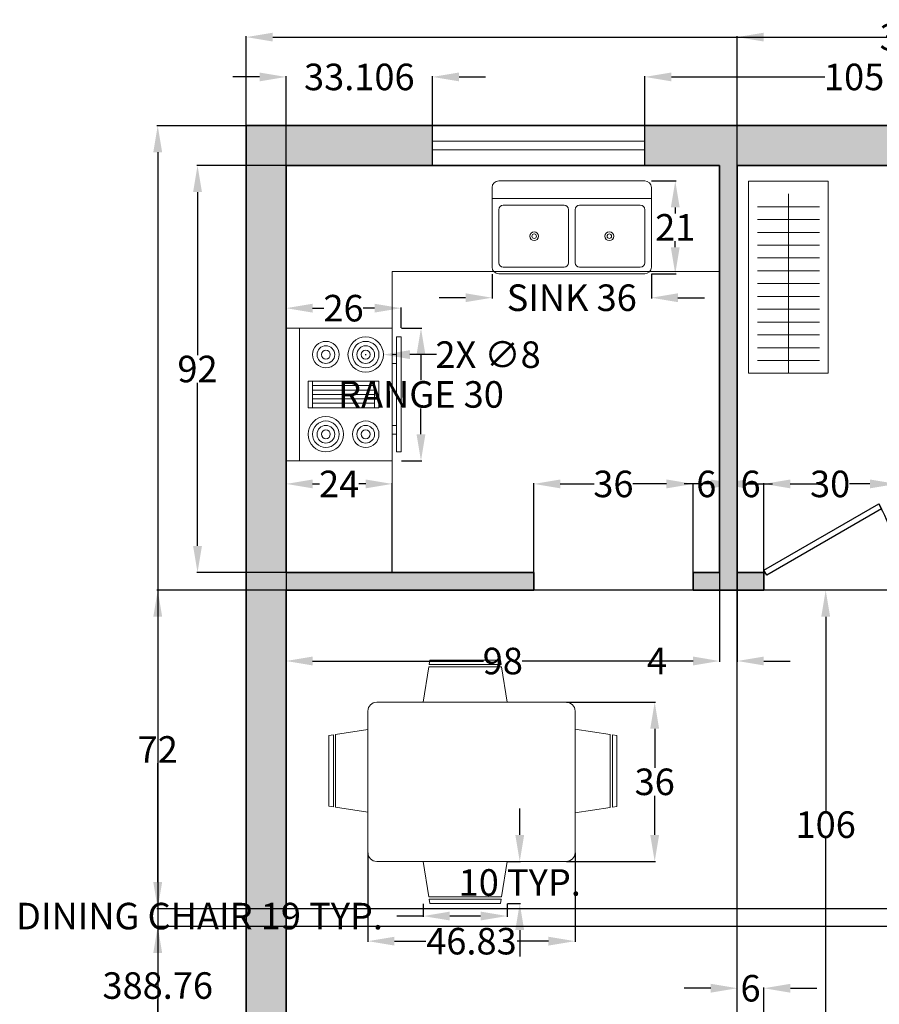
# Model space of a CAD drawing. Units: inches. Extents: x -26 to 363, y -399 to 37.
# Tile 3 of 4: x -26 to 168, y -185 to 37. Entities that reach past the tile are written whole.
import ezdxf

# ---------------------------------------------------------------- set-up
doc = ezdxf.new("R2010")
doc.units = ezdxf.units.IN
doc.header["$MEASUREMENT"] = 0
for name, color, linetype, lineweight in [('A-ANNO-DIMS', 2, 'Continuous', 18), ('A-DOOR', 3, 'Continuous', 25), ('A-EQPM', 9, 'Continuous', 18), ('A-FLOR-CASE', 8, 'Continuous', 18), ('A-FLOR-FIXT', 9, 'Continuous', 18), ('A-FURN', 8, 'Continuous', 18), ('A-GLAZ', 4, 'Continuous', 18), ('A-WALL', 7, 'Continuous', 35), ('A-WALL-PATT', 251, 'Continuous', 13)]:
    doc.layers.add(name, color=color, linetype=linetype, lineweight=lineweight)
doc.styles.get("Standard").update_dxf_attribs({"font": 'arial.ttf'})
doc.dimstyles.get("Standard").update_dxf_attribs({"dimtxt": 6, "dimasz": 6, "dimexe": 0.18, "dimexo": 0.0625, "dimgap": 0.09, "dimtad": 0, "dimtih": 1, "dimtoh": 1, "dimdec": 0, "dimzin": 0, "dimdsep": 46, "dimlunit": 4, "dimtxsty": 'Standard', "dimcen": 0.09, "dimadec": 0, "dimazin": 0, "dimtfac": 1, "dimtdec": 0, "dimtofl": 0, "dimtmove": 0, "dimatfit": 3, "dimfxl": 1, "dimtolj": 1, "dimtzin": 0, "dimarcsym": 0})

# ---------------------------------------------------------------- blocks, each defined once
blk = doc.blocks.new('*U2')
for p, q in [((0, 0), (0, -6)), ((40, 0), (40, -6))]:
    blk.add_line(p, q)
blk.add_lwpolyline([(0, 0), (34.64, 20), (35.52, 18.48), (0.87, -1.52)], close=True)
blk.add_arc((0, 0), 40, 0, 30)
blk = doc.blocks.new('Range-Oven - 30 in top')
for p, q in [((0, -3), (30, -3)), ((12, -6), (18, -6)), ((13, -20), (13, -6)), ((14, -6), (14, -20)), ((15, -20), (15, -6)), ((16, -6), (16, -20)), ((17, -20), (17, -6)), ((18, -20), (12, -20)), ((6, -24), (6, -25)), ((8, -25), (8, -24)), ((22, -25), (22, -24)), ((24, -24), (24, -25))]:
    blk.add_line(p, q)
for points in [[(0, -24), (0, 0), (30, 0), (30, -24)], [(12, -21), (12, -5), (18, -5), (18, -21)], [(2, -26), (2, -25), (28, -25), (28, -26)]]:
    blk.add_lwpolyline(points, close=True)
for centre, radius in [((6, -9), 4), ((6, -9), 3), ((24, -9), 3), ((6, -9), 2), ((6, -9), 1), ((24, -9), 2), ((24, -9), 1), ((6, -18), 3), ((24, -18), 4), ((24, -18), 3), ((6, -18), 2), ((6, -18), 1), ((24, -18), 2), ((24, -18), 1)]:
    blk.add_circle(centre, radius)
blk = doc.blocks.new('Sink-double - 36 in top')
for p, q in [((-18, -4), (18, -4)), ((-0.75, -18.5), (-0.75, -6.5)), ((0.75, -6.5), (0.75, -18.5))]:
    blk.add_line(p, q)
for points in [[(-16.5, 0), (16.5, 0)], [(-18, -19.5), (-18, -1.5)], [(18, -1.5), (18, -19.5)], [(-16.5, -18.5), (-16.5, -6.5)], [(-15.5, -5.5), (-1.75, -5.5)], [(1.75, -5.5), (15.5, -5.5)], [(16.5, -6.5), (16.5, -18.5)], [(-1.75, -19.5), (-15.5, -19.5)], [(15.5, -19.5), (1.75, -19.5)], [(16.5, -21), (-16.5, -21)]]:
    blk.add_lwpolyline(points)
for centre, radius in [((-8.5, -12.5), 1), ((-8.5, -12.5), 0.5), ((8.5, -12.5), 1), ((8.5, -12.5), 0.5)]:
    blk.add_circle(centre, radius)
for centre, radius, start, end in [((-16.5, -1.5), 1.5, 90, 180), ((16.5, -1.5), 1.5, 0, 90), ((-15.5, -6.5), 1, 90, 180), ((-1.75, -6.5), 1, 0, 90), ((1.75, -6.5), 1, 90, 180), ((15.5, -6.5), 1, 0, 90), ((-16.5, -19.5), 1.5, 180, 270), ((-15.5, -18.5), 1, 180, 270), ((-1.75, -18.5), 1, 270, 0), ((1.75, -18.5), 1, 180, 270), ((15.5, -18.5), 1, 270, 0), ((16.5, -19.5), 1.5, 270, 0)]:
    blk.add_arc(centre, radius, start, end)
blk = doc.blocks.new('WIN-48IN')
for p, q in [((0, 0), (0, 9)), ((48, 9), (48, 0)), ((48, 5.5), (0, 5.5)), ((48, 3.5), (0, 3.5))]:
    blk.add_line(p, q)
blk = doc.blocks.new('CHAIR-DINING')
for p, q in [((1.48, 9.5), (1.33, 8.5)), ((1.48, 9.5), (17.48, 9.5)), ((17.64, 8.5), (17.48, 9.5)), ((1.25, 8), (0, 0)), ((1.25, 8), (17.72, 8)), ((17.64, 8.5), (1.33, 8.5)), ((18.97, 0), (17.72, 8))]:
    blk.add_line(p, q)
blk = doc.blocks.new('*D25')
at = {"layer": 'A-ANNO-DIMS', "color": 0, "lineweight": -2, "transparency": 16777216}
for p, q in [((65.33, -162.44), (65.33, -165.41)), ((84.3, -162.44), (84.3, -165.4)), ((65.33, -165.23), (59.33, -165.23)), ((78.3, -165.22), (71.33, -165.22))]:
    blk.add_line(p, q, dxfattribs=at)
at = {"layer": 'A-ANNO-DIMS', "color": 0, "transparency": 16777216}
for points in [[(71.33, -164.22), (71.33, -166.22), (65.33, -165.23)], [(78.3, -164.22), (78.3, -166.22), (84.3, -165.22)]]:
    blk.add_solid(points, dxfattribs=at)
at = {"layer": 'Defpoints', "color": 0, "transparency": 16777216}
for p in [(65.33, -162.38), (84.3, -162.38), (65.33, -165.23)]:
    blk.add_point(p, dxfattribs=at)
at = {"layer": 'A-ANNO-DIMS', "color": 0, "transparency": 16777216, "insert": (14.75, -165.23), "char_height": 6, "attachment_point": 5}
blk.add_mtext('\\A1;DINING CHAIR 19 TYP.', dxfattribs=at)
blk = doc.blocks.new('*D26')
at = {"layer": 'A-ANNO-DIMS', "color": 0, "lineweight": -2, "transparency": 16777216}
for p, q in [((87.15, -146.88), (87.15, -140.88)), ((84.36, -152.88), (87.33, -152.88)), ((84.36, -162.38), (87.33, -162.38)), ((87.15, -168.38), (87.15, -174.38))]:
    blk.add_line(p, q, dxfattribs=at)
at = {"layer": 'A-ANNO-DIMS', "color": 0, "transparency": 16777216}
for points in [[(88.15, -146.88), (86.15, -146.88), (87.15, -152.88)], [(88.15, -168.38), (86.15, -168.38), (87.15, -162.38)]]:
    blk.add_solid(points, dxfattribs=at)
at = {"layer": 'Defpoints', "color": 0, "transparency": 16777216}
for p in [(84.3, -152.88), (84.3, -162.38), (87.15, -162.38)]:
    blk.add_point(p, dxfattribs=at)
at = {"layer": 'A-ANNO-DIMS', "color": 0, "transparency": 16777216, "insert": (87.15, -157.63), "char_height": 6, "attachment_point": 5}
blk.add_mtext('\\A1;10 TYP.', dxfattribs=at)
blk = doc.blocks.new('*D33')
at = {"layer": 'A-ANNO-DIMS', "color": 0, "lineweight": -2, "transparency": 16777216}
for p, q in [((60.39, -32.31), (65, -32.31)), ((64.82, -38.31), (64.82, -44.12)), ((64.82, -56.31), (64.82, -50.51)), ((60.39, -62.31), (65, -62.31))]:
    blk.add_line(p, q, dxfattribs=at)
at = {"layer": 'A-ANNO-DIMS', "color": 0, "transparency": 16777216}
for points in [[(63.82, -38.31), (65.82, -38.31), (64.82, -32.31)], [(63.82, -56.31), (65.82, -56.31), (64.82, -62.31)]]:
    blk.add_solid(points, dxfattribs=at)
at = {"layer": 'Defpoints', "color": 0, "transparency": 16777216}
for p in [(60.32, -32.31), (64.82, -32.31), (60.32, -62.31)]:
    blk.add_point(p, dxfattribs=at)
at = {"layer": 'A-ANNO-DIMS', "color": 0, "transparency": 16777216, "insert": (64.82, -47.31), "char_height": 6, "attachment_point": 5}
blk.add_mtext('\\A1;RANGE 30', dxfattribs=at)
blk = doc.blocks.new('*D34')
at = {"layer": 'A-ANNO-DIMS', "color": 0, "lineweight": -2, "transparency": 16777216}
for p, q in [((34.32, -32.25), (34.32, -27.63)), ((40.32, -27.81), (42.89, -27.81)), ((54.32, -27.81), (51.76, -27.81)), ((60.32, -32.25), (60.32, -27.63))]:
    blk.add_line(p, q, dxfattribs=at)
at = {"layer": 'A-ANNO-DIMS', "color": 0, "transparency": 16777216}
for points in [[(40.32, -26.81), (40.32, -28.81), (34.32, -27.81)], [(54.32, -26.81), (54.32, -28.81), (60.32, -27.81)]]:
    blk.add_solid(points, dxfattribs=at)
at = {"layer": 'Defpoints', "color": 0, "transparency": 16777216}
for p in [(34.32, -27.81), (34.32, -32.31), (60.32, -32.31)]:
    blk.add_point(p, dxfattribs=at)
at = {"layer": 'A-ANNO-DIMS', "color": 0, "transparency": 16777216, "insert": (47.32, -27.81), "char_height": 6, "attachment_point": 5}
blk.add_mtext('\\A1;26', dxfattribs=at)
blk = doc.blocks.new('*D35')
at = {"layer": 'A-ANNO-DIMS', "color": 0, "lineweight": -2, "transparency": 16777216}
for p, q in [((80.91, -20.11), (80.91, -25.63)), ((116.91, -20.11), (116.91, -25.63)), ((74.91, -25.45), (68.91, -25.45)), ((122.91, -25.45), (128.91, -25.45))]:
    blk.add_line(p, q, dxfattribs=at)
at = {"layer": 'A-ANNO-DIMS', "color": 0, "transparency": 16777216}
for points in [[(74.91, -24.45), (74.91, -26.45), (80.91, -25.45)], [(122.91, -24.45), (122.91, -26.45), (116.91, -25.45)]]:
    blk.add_solid(points, dxfattribs=at)
at = {"layer": 'Defpoints', "color": 0, "transparency": 16777216}
for p in [(80.91, -20.05), (116.91, -20.05), (116.91, -25.45)]:
    blk.add_point(p, dxfattribs=at)
at = {"layer": 'A-ANNO-DIMS', "color": 0, "transparency": 16777216, "insert": (98.91, -25.45), "char_height": 6, "attachment_point": 5}
blk.add_mtext('\\A1;SINK 36', dxfattribs=at)
blk = doc.blocks.new('*D36')
at = {"layer": 'A-ANNO-DIMS', "color": 0, "lineweight": -2, "transparency": 16777216}
for p, q in [((116.97, 0.95), (122.49, 0.95)), ((122.31, -5.05), (122.31, -6.44)), ((122.31, -14.05), (122.31, -12.65)), ((116.97, -20.05), (122.49, -20.05))]:
    blk.add_line(p, q, dxfattribs=at)
at = {"layer": 'A-ANNO-DIMS', "color": 0, "transparency": 16777216}
for points in [[(121.31, -5.05), (123.31, -5.05), (122.31, 0.95)], [(121.31, -14.05), (123.31, -14.05), (122.31, -20.05)]]:
    blk.add_solid(points, dxfattribs=at)
at = {"layer": 'Defpoints', "color": 0, "transparency": 16777216}
for p in [(116.91, 0.95), (122.31, 0.95), (116.91, -20.05)]:
    blk.add_point(p, dxfattribs=at)
at = {"layer": 'A-ANNO-DIMS', "color": 0, "transparency": 16777216, "insert": (122.31, -9.55), "char_height": 6, "attachment_point": 5}
blk.add_mtext('\\A1;21', dxfattribs=at)
blk = doc.blocks.new('*D39')
at = {"layer": 'A-ANNO-DIMS', "color": 0, "lineweight": -2, "transparency": 16777216}
for p, q in [((25.32, 13.51), (25.32, 33.64)), ((31.32, 33.46), (168.62, 33.46)), ((319.32, 33.46), (182.03, 33.46)), ((325.32, 13.51), (325.32, 33.64))]:
    blk.add_line(p, q, dxfattribs=at)
at = {"layer": 'A-ANNO-DIMS', "color": 0, "transparency": 16777216}
for points in [[(31.32, 34.46), (31.32, 32.46), (25.32, 33.46)], [(319.32, 34.46), (319.32, 32.46), (325.32, 33.46)]]:
    blk.add_solid(points, dxfattribs=at)
at = {"layer": 'Defpoints', "color": 0, "transparency": 16777216}
for p in [(325.32, 33.46), (25.32, 13.44), (325.32, 13.44)]:
    blk.add_point(p, dxfattribs=at)
at = {"layer": 'A-ANNO-DIMS', "color": 0, "transparency": 16777216, "insert": (175.32, 33.46), "char_height": 6, "attachment_point": 5}
blk.add_mtext('\\A1;300', dxfattribs=at)
blk = doc.blocks.new('*D40')
at = {"layer": 'A-ANNO-DIMS', "color": 0, "lineweight": -2, "transparency": 16777216}
for p, q in [((25.26, 13.44), (5.13, 13.44)), ((5.31, 7.44), (5.31, -177.78)), ((5.31, -369.31), (5.31, -184.09)), ((76.26, -375.31), (5.13, -375.31))]:
    blk.add_line(p, q, dxfattribs=at)
at = {"layer": 'A-ANNO-DIMS', "color": 0, "transparency": 16777216}
for points in [[(4.31, 7.44), (6.31, 7.44), (5.31, 13.44)], [(4.31, -369.31), (6.31, -369.31), (5.31, -375.31)]]:
    blk.add_solid(points, dxfattribs=at)
at = {"layer": 'Defpoints', "color": 0, "transparency": 16777216}
for p in [(25.32, 13.44), (5.31, -375.31), (76.32, -375.31)]:
    blk.add_point(p, dxfattribs=at)
at = {"layer": 'A-ANNO-DIMS', "color": 0, "transparency": 16777216, "insert": (5.31, -180.93), "char_height": 6, "attachment_point": 5}
blk.add_mtext('\\A1;388.76', dxfattribs=at)
blk = doc.blocks.new('*D45')
at = {"layer": 'A-ANNO-DIMS', "color": 0, "lineweight": -2, "transparency": 16777216}
for p, q in [((34.32, -87.62), (34.32, -107.75)), ((132.32, -87.62), (132.32, -107.75)), ((40.32, -107.57), (78.93, -107.57)), ((126.32, -107.57), (87.72, -107.57))]:
    blk.add_line(p, q, dxfattribs=at)
at = {"layer": 'A-ANNO-DIMS', "color": 0, "transparency": 16777216}
for points in [[(40.32, -106.57), (40.32, -108.57), (34.32, -107.57)], [(126.32, -106.57), (126.32, -108.57), (132.32, -107.57)]]:
    blk.add_solid(points, dxfattribs=at)
at = {"layer": 'Defpoints', "color": 0, "transparency": 16777216}
for p in [(34.32, -87.56), (132.32, -87.56), (34.32, -107.57)]:
    blk.add_point(p, dxfattribs=at)
at = {"layer": 'A-ANNO-DIMS', "color": 0, "transparency": 16777216, "insert": (83.32, -107.57), "char_height": 6, "attachment_point": 5}
blk.add_mtext('\\A1;98', dxfattribs=at)
blk = doc.blocks.new('*D46')
at = {"layer": 'A-ANNO-DIMS', "color": 0, "lineweight": -2, "transparency": 16777216}
for p, q in [((34.26, 4.44), (14.13, 4.44)), ((14.31, -1.56), (14.31, -38.4)), ((14.31, -81.56), (14.31, -44.71)), ((34.26, -87.56), (14.13, -87.56))]:
    blk.add_line(p, q, dxfattribs=at)
at = {"layer": 'A-ANNO-DIMS', "color": 0, "transparency": 16777216}
for points in [[(13.31, -1.56), (15.31, -1.56), (14.31, 4.44)], [(13.31, -81.56), (15.31, -81.56), (14.31, -87.56)]]:
    blk.add_solid(points, dxfattribs=at)
at = {"layer": 'Defpoints', "color": 0, "transparency": 16777216}
for p in [(14.31, 4.44), (34.32, 4.44), (34.32, -87.56)]:
    blk.add_point(p, dxfattribs=at)
at = {"layer": 'A-ANNO-DIMS', "color": 0, "transparency": 16777216, "insert": (14.31, -41.56), "char_height": 6, "attachment_point": 5}
blk.add_mtext('\\A1;92', dxfattribs=at)
blk = doc.blocks.new('*D48')
at = {"layer": 'A-ANNO-DIMS', "color": 0, "lineweight": -2, "transparency": 16777216}
for p, q in [((176.26, -91.56), (156.13, -91.56)), ((156.31, -97.56), (156.31, -141.4)), ((156.31, -191.56), (156.31, -147.71)), ((176.26, -197.56), (156.13, -197.56))]:
    blk.add_line(p, q, dxfattribs=at)
at = {"layer": 'A-ANNO-DIMS', "color": 0, "transparency": 16777216}
for points in [[(155.31, -97.56), (157.31, -97.56), (156.31, -91.56)], [(155.31, -191.56), (157.31, -191.56), (156.31, -197.56)]]:
    blk.add_solid(points, dxfattribs=at)
at = {"layer": 'Defpoints', "color": 0, "transparency": 16777216}
for p in [(156.31, -91.56), (176.32, -91.56), (176.32, -197.56)]:
    blk.add_point(p, dxfattribs=at)
at = {"layer": 'A-ANNO-DIMS', "color": 0, "transparency": 16777216, "insert": (156.31, -144.56), "char_height": 6, "attachment_point": 5}
blk.add_mtext('\\A1;106', dxfattribs=at)
blk = doc.blocks.new('*D50')
at = {"layer": 'A-ANNO-DIMS', "color": 0, "lineweight": -2, "transparency": 16777216}
for p, q in [((268.26, -91.56), (5.13, -91.56)), ((5.31, -97.56), (5.31, -124.45)), ((5.31, -157.56), (5.31, -130.66)), ((268.26, -163.56), (5.13, -163.56))]:
    blk.add_line(p, q, dxfattribs=at)
at = {"layer": 'A-ANNO-DIMS', "color": 0, "transparency": 16777216}
for points in [[(4.31, -97.56), (6.31, -97.56), (5.31, -91.56)], [(4.31, -157.56), (6.31, -157.56), (5.31, -163.56)]]:
    blk.add_solid(points, dxfattribs=at)
at = {"layer": 'Defpoints', "color": 0, "transparency": 16777216}
for p in [(268.32, -91.56), (5.31, -163.56), (268.32, -163.56)]:
    blk.add_point(p, dxfattribs=at)
at = {"layer": 'A-ANNO-DIMS', "color": 0, "transparency": 16777216, "insert": (5.31, -127.56), "char_height": 6, "attachment_point": 5}
blk.add_mtext('\\A1;72', dxfattribs=at)
blk = doc.blocks.new('*D51')
at = {"layer": 'A-ANNO-DIMS', "color": 0, "lineweight": -2, "transparency": 16777216}
for p, q in [((268.26, -167.56), (5.13, -167.56)), ((5.31, -173.56), (5.31, -196.4)), ((5.31, -225.56), (5.31, -202.71)), ((268.26, -231.56), (5.13, -231.56))]:
    blk.add_line(p, q, dxfattribs=at)
at = {"layer": 'A-ANNO-DIMS', "color": 0, "transparency": 16777216}
for points in [[(4.31, -173.56), (6.31, -173.56), (5.31, -167.56)], [(4.31, -225.56), (6.31, -225.56), (5.31, -231.56)]]:
    blk.add_solid(points, dxfattribs=at)
at = {"layer": 'Defpoints', "color": 0, "transparency": 16777216}
for p in [(268.32, -167.56), (5.31, -231.56), (268.32, -231.56)]:
    blk.add_point(p, dxfattribs=at)
at = {"layer": 'A-ANNO-DIMS', "color": 0, "transparency": 16777216, "insert": (5.31, -199.56), "char_height": 6, "attachment_point": 5}
blk.add_mtext('\\A1;64', dxfattribs=at)
blk = doc.blocks.new('*D53')
at = {"layer": 'A-ANNO-DIMS', "color": 0, "lineweight": -2, "transparency": 16777216}
for p, q in [((34.32, 4.51), (34.32, 24.64)), ((67.43, 4.51), (67.43, 24.64)), ((28.32, 24.46), (22.32, 24.46)), ((73.43, 24.46), (79.43, 24.46))]:
    blk.add_line(p, q, dxfattribs=at)
at = {"layer": 'A-ANNO-DIMS', "color": 0, "transparency": 16777216}
for points in [[(28.32, 25.46), (28.32, 23.46), (34.32, 24.46)], [(73.43, 25.46), (73.43, 23.46), (67.43, 24.46)]]:
    blk.add_solid(points, dxfattribs=at)
at = {"layer": 'Defpoints', "color": 0, "transparency": 16777216}
for p in [(67.43, 24.46), (34.32, 4.44), (67.43, 4.44)]:
    blk.add_point(p, dxfattribs=at)
at = {"layer": 'A-ANNO-DIMS', "color": 0, "transparency": 16777216, "insert": (50.88, 24.46), "char_height": 6, "attachment_point": 5}
blk.add_mtext('\\A1;33.106', dxfattribs=at)
blk = doc.blocks.new('*D54')
at = {"layer": 'A-ANNO-DIMS', "color": 0, "lineweight": -2, "transparency": 16777216}
for p, q in [((115.43, 4.51), (115.43, 24.64)), ((221.4, 4.51), (221.4, 24.64)), ((121.43, 24.46), (156.15, 24.46)), ((215.4, 24.46), (180.68, 24.46))]:
    blk.add_line(p, q, dxfattribs=at)
at = {"layer": 'A-ANNO-DIMS', "color": 0, "transparency": 16777216}
for points in [[(121.43, 25.46), (121.43, 23.46), (115.43, 24.46)], [(215.4, 25.46), (215.4, 23.46), (221.4, 24.46)]]:
    blk.add_solid(points, dxfattribs=at)
at = {"layer": 'Defpoints', "color": 0, "transparency": 16777216}
for p in [(221.4, 24.46), (115.43, 4.44), (221.4, 4.44)]:
    blk.add_point(p, dxfattribs=at)
at = {"layer": 'A-ANNO-DIMS', "color": 0, "transparency": 16777216, "insert": (168.42, 24.46), "char_height": 6, "attachment_point": 5}
blk.add_mtext('\\A1;105.98', dxfattribs=at)
blk = doc.blocks.new('*D60')
at = {"layer": 'A-ANNO-DIMS', "color": 0, "lineweight": -2, "transparency": 16777216}
for p, q in [((90.32, -87.49), (90.32, -67.36)), ((96.32, -67.54), (103.94, -67.54)), ((120.32, -67.54), (112.71, -67.54)), ((126.32, -87.49), (126.32, -67.36))]:
    blk.add_line(p, q, dxfattribs=at)
at = {"layer": 'A-ANNO-DIMS', "color": 0, "transparency": 16777216}
for points in [[(96.32, -66.54), (96.32, -68.54), (90.32, -67.54)], [(120.32, -66.54), (120.32, -68.54), (126.32, -67.54)]]:
    blk.add_solid(points, dxfattribs=at)
at = {"layer": 'Defpoints', "color": 0, "transparency": 16777216}
for p in [(126.32, -67.54), (90.32, -87.56), (126.32, -87.56)]:
    blk.add_point(p, dxfattribs=at)
at = {"layer": 'A-ANNO-DIMS', "color": 0, "transparency": 16777216, "insert": (108.32, -67.54), "char_height": 6, "attachment_point": 5}
blk.add_mtext('\\A1;36', dxfattribs=at)
blk = doc.blocks.new('*D61')
at = {"layer": 'A-ANNO-DIMS', "color": 0, "lineweight": -2, "transparency": 16777216}
for p, q in [((142.32, -87.49), (142.32, -67.36)), ((148.32, -67.54), (152.95, -67.54)), ((166.32, -67.54), (161.7, -67.54)), ((172.32, -87.49), (172.32, -67.36))]:
    blk.add_line(p, q, dxfattribs=at)
at = {"layer": 'A-ANNO-DIMS', "color": 0, "transparency": 16777216}
for points in [[(148.32, -66.54), (148.32, -68.54), (142.32, -67.54)], [(166.32, -66.54), (166.32, -68.54), (172.32, -67.54)]]:
    blk.add_solid(points, dxfattribs=at)
at = {"layer": 'Defpoints', "color": 0, "transparency": 16777216}
for p in [(172.32, -67.54), (142.32, -87.56), (172.32, -87.56)]:
    blk.add_point(p, dxfattribs=at)
at = {"layer": 'A-ANNO-DIMS', "color": 0, "transparency": 16777216, "insert": (157.32, -67.54), "char_height": 6, "attachment_point": 5}
blk.add_mtext('\\A1;30', dxfattribs=at)
blk = doc.blocks.new('*D71')
at = {"layer": 'A-ANNO-DIMS', "color": 0, "lineweight": -2, "transparency": 16777216}
for p, q in [((130.322775, -181.538613), (124.322775, -181.538613)), ((136.322775, -201.492613), (136.322775, -181.358613)), ((142.322775, -201.492613), (142.322775, -181.358613)), ((148.322775, -181.538613), (154.322775, -181.538613))]:
    blk.add_line(p, q, dxfattribs=at)
at = {"layer": 'A-ANNO-DIMS', "color": 0, "transparency": 16777216}
for points in [[(130.322775, -180.538613), (130.322775, -182.538613), (136.322775, -181.538613)], [(148.322775, -180.538613), (148.322775, -182.538613), (142.322775, -181.538613)]]:
    blk.add_solid(points, dxfattribs=at)
at = {"layer": 'Defpoints', "color": 0, "transparency": 16777216}
for p in [(142.322775, -181.538613), (136.322775, -201.555113), (142.322775, -201.555113)]:
    blk.add_point(p, dxfattribs=at)
at = {"layer": 'A-ANNO-DIMS', "color": 0, "transparency": 16777216, "insert": (139.322775, -181.538613), "char_height": 6, "attachment_point": 5}
blk.add_mtext('\\A1;6', dxfattribs=at)
blk = doc.blocks.new('*D72')
at = {"layer": 'A-ANNO-DIMS', "color": 0, "lineweight": -2, "transparency": 16777216}
for p, q in [((34.32, -87.49), (34.32, -67.36)), ((40.32, -67.54), (41.9, -67.54)), ((52.32, -67.54), (50.75, -67.54)), ((58.32, -87.49), (58.32, -67.36))]:
    blk.add_line(p, q, dxfattribs=at)
at = {"layer": 'A-ANNO-DIMS', "color": 0, "transparency": 16777216}
for points in [[(40.32, -66.54), (40.32, -68.54), (34.32, -67.54)], [(52.32, -66.54), (52.32, -68.54), (58.32, -67.54)]]:
    blk.add_solid(points, dxfattribs=at)
at = {"layer": 'Defpoints', "color": 0, "transparency": 16777216}
for p in [(58.32, -67.54), (34.32, -87.56), (58.32, -87.56)]:
    blk.add_point(p, dxfattribs=at)
at = {"layer": 'A-ANNO-DIMS', "color": 0, "transparency": 16777216, "insert": (46.32, -67.54), "char_height": 6, "attachment_point": 5}
blk.add_mtext('\\A1;24', dxfattribs=at)
blk = doc.blocks.new('*D73')
at = {"layer": 'A-ANNO-DIMS', "color": 0, "lineweight": -2, "transparency": 16777216}
for p, q in [((52.82, -150.94), (52.82, -171.08)), ((99.65, -150.94), (99.65, -171.08)), ((58.82, -170.9), (65.9, -170.9)), ((93.65, -170.9), (86.57, -170.9))]:
    blk.add_line(p, q, dxfattribs=at)
at = {"layer": 'A-ANNO-DIMS', "color": 0, "transparency": 16777216}
for points in [[(58.82, -169.9), (58.82, -171.9), (52.82, -170.9)], [(93.65, -169.9), (93.65, -171.9), (99.65, -170.9)]]:
    blk.add_solid(points, dxfattribs=at)
at = {"layer": 'Defpoints', "color": 0, "transparency": 16777216}
for p in [(52.82, -150.88), (99.65, -150.88), (52.82, -170.9)]:
    blk.add_point(p, dxfattribs=at)
at = {"layer": 'A-ANNO-DIMS', "color": 0, "transparency": 16777216, "insert": (76.23, -170.9), "char_height": 6, "attachment_point": 5}
blk.add_mtext('\\A1;46.83', dxfattribs=at)
blk = doc.blocks.new('*D74')
at = {"layer": 'A-ANNO-DIMS', "color": 0, "lineweight": -2, "transparency": 16777216}
for p, q in [((97.71, -116.88), (117.84, -116.88)), ((117.66, -122.88), (117.66, -131.72)), ((117.66, -146.88), (117.66, -138.03)), ((97.71, -152.88), (117.84, -152.88))]:
    blk.add_line(p, q, dxfattribs=at)
at = {"layer": 'A-ANNO-DIMS', "color": 0, "transparency": 16777216}
for points in [[(116.66, -122.88), (118.66, -122.88), (117.66, -116.88)], [(116.66, -146.88), (118.66, -146.88), (117.66, -152.88)]]:
    blk.add_solid(points, dxfattribs=at)
at = {"layer": 'Defpoints', "color": 0, "transparency": 16777216}
for p in [(97.65, -116.88), (97.65, -152.88), (117.66, -152.88)]:
    blk.add_point(p, dxfattribs=at)
at = {"layer": 'A-ANNO-DIMS', "color": 0, "transparency": 16777216, "insert": (117.66, -134.88), "char_height": 6, "attachment_point": 5}
blk.add_mtext('\\A1;36', dxfattribs=at)
blk = doc.blocks.new('*D76')
at = {"layer": 'A-ANNO-DIMS', "color": 0, "lineweight": -2, "transparency": 16777216}
for p, q in [((136.32, -337.49), (136.32, 33.64)), ((142.32, 33.46), (178.95, 33.46)), ((224.32, 33.46), (187.7, 33.46)), ((230.32, -337.49), (230.32, 33.64))]:
    blk.add_line(p, q, dxfattribs=at)
at = {"layer": 'A-ANNO-DIMS', "color": 0, "transparency": 16777216}
for points in [[(142.32, 34.46), (142.32, 32.46), (136.32, 33.46)], [(224.32, 34.46), (224.32, 32.46), (230.32, 33.46)]]:
    blk.add_solid(points, dxfattribs=at)
at = {"layer": 'Defpoints', "color": 0, "transparency": 16777216}
for p in [(230.32, 33.46), (136.32, -337.56), (230.32, -337.56)]:
    blk.add_point(p, dxfattribs=at)
at = {"layer": 'A-ANNO-DIMS', "color": 0, "transparency": 16777216, "insert": (183.32, 33.46), "char_height": 6, "attachment_point": 5}
blk.add_mtext('\\A1;94', dxfattribs=at)
blk = doc.blocks.new('*D79')
at = {"layer": 'A-ANNO-DIMS', "color": 0, "lineweight": -2, "transparency": 16777216}
for p, q in [((132.32, -87.62), (132.32, -107.75)), ((136.32, -87.62), (136.32, -107.75)), ((126.32, -107.57), (120.32, -107.57)), ((142.32, -107.57), (148.32, -107.57))]:
    blk.add_line(p, q, dxfattribs=at)
at = {"layer": 'A-ANNO-DIMS', "color": 0, "transparency": 16777216}
for points in [[(126.32, -106.57), (126.32, -108.57), (132.32, -107.57)], [(142.32, -106.57), (142.32, -108.57), (136.32, -107.57)]]:
    blk.add_solid(points, dxfattribs=at)
at = {"layer": 'Defpoints', "color": 0, "transparency": 16777216}
for p in [(132.32, -87.56), (136.32, -87.56), (132.32, -107.57)]:
    blk.add_point(p, dxfattribs=at)
at = {"layer": 'A-ANNO-DIMS', "color": 0, "transparency": 16777216, "insert": (118.16, -107.57), "char_height": 6, "attachment_point": 5}
blk.add_mtext('\\A1;4', dxfattribs=at)
blk = doc.blocks.new('*D80')
at = {"layer": 'A-ANNO-DIMS', "color": 0, "lineweight": -2, "transparency": 16777216}
for p, q in [((120.322775, -67.538613), (114.322775, -67.538613)), ((126.322775, -87.492613), (126.322775, -67.358613)), ((132.322775, -87.492613), (132.322775, -67.358613)), ((138.322775, -67.538613), (144.322775, -67.538613))]:
    blk.add_line(p, q, dxfattribs=at)
at = {"layer": 'A-ANNO-DIMS', "color": 0, "transparency": 16777216}
for points in [[(120.322775, -66.538613), (120.322775, -68.538613), (126.322775, -67.538613)], [(138.322775, -66.538613), (138.322775, -68.538613), (132.322775, -67.538613)]]:
    blk.add_solid(points, dxfattribs=at)
at = {"layer": 'Defpoints', "color": 0, "transparency": 16777216}
for p in [(132.322775, -67.538613), (126.322775, -87.555113), (132.322775, -87.555113)]:
    blk.add_point(p, dxfattribs=at)
at = {"layer": 'A-ANNO-DIMS', "color": 0, "transparency": 16777216, "insert": (129.322775, -67.538613), "char_height": 6, "attachment_point": 5}
blk.add_mtext('\\A1;6', dxfattribs=at)
blk = doc.blocks.new('*D81')
at = {"layer": 'A-ANNO-DIMS', "color": 0, "lineweight": -2, "transparency": 16777216}
for p, q in [((130.322775, -67.538613), (124.322775, -67.538613)), ((136.322775, -87.492613), (136.322775, -67.358613)), ((142.322775, -87.492613), (142.322775, -67.358613)), ((148.322775, -67.538613), (154.322775, -67.538613))]:
    blk.add_line(p, q, dxfattribs=at)
at = {"layer": 'A-ANNO-DIMS', "color": 0, "transparency": 16777216}
for points in [[(130.322775, -66.538613), (130.322775, -68.538613), (136.322775, -67.538613)], [(148.322775, -66.538613), (148.322775, -68.538613), (142.322775, -67.538613)]]:
    blk.add_solid(points, dxfattribs=at)
at = {"layer": 'Defpoints', "color": 0, "transparency": 16777216}
for p in [(142.322775, -67.538613), (136.322775, -87.555113), (142.322775, -87.555113)]:
    blk.add_point(p, dxfattribs=at)
at = {"layer": 'A-ANNO-DIMS', "color": 0, "transparency": 16777216, "insert": (139.322775, -67.538613), "char_height": 6, "attachment_point": 5}
blk.add_mtext('\\A1;6', dxfattribs=at)
blk = doc.blocks.new('*D85')
at = {"layer": 'A-ANNO-DIMS', "color": 0, "lineweight": -2, "transparency": 16777216}
for p, q in [((52.23, -38.31), (52.41, -38.31)), ((52.32, -38.4), (52.32, -38.22)), ((68.32, -38.31), (62.32, -38.31))]:
    blk.add_line(p, q, dxfattribs=at)
at = {"layer": 'A-ANNO-DIMS', "color": 0, "transparency": 16777216}
blk.add_solid([(62.32, -37.31), (62.32, -39.31), (56.32, -38.31)], dxfattribs=at)
at = {"layer": 'Defpoints', "color": 0, "transparency": 16777216}
for p in [(48.32, -38.31), (56.32, -38.31)]:
    blk.add_point(p, dxfattribs=at)
at = {"layer": 'A-ANNO-DIMS', "color": 0, "transparency": 16777216, "insert": (79.99, -38.31), "char_height": 6, "attachment_point": 5}
blk.add_mtext('\\A1;2X ∅8', dxfattribs=at)

msp = doc.modelspace()

# ---------------------------------------------------------------- hatches: boundary and pattern name
at = {"layer": 'A-WALL-PATT'}
h = msp.add_hatch(color=256, dxfattribs=at)
h.dxf.hatch_style = 1
h.paths.add_polyline_path([(34.3228, -91.5551), (90.3228, -91.5551), (90.3228, -87.5551), (34.3228, -87.5551), (34.3228, 4.4449), (67.429, 4.4449), (67.429, 13.4449), (25.3228, 13.4449), (25.3228, -315.3126), (34.3228, -315.3126), (40.3228, -315.3126), (40.3228, -306.3126), (34.3228, -306.3126)])
h = msp.add_hatch(color=256, dxfattribs=at)
h.dxf.hatch_style = 1
h.paths.add_polyline_path([(221.4046, 13.4449), (115.429, 13.4449), (115.429, 4.4449), (132.3228, 4.4449), (132.3228, -87.5551), (126.3228, -87.5551), (126.3228, -91.5551), (142.3228, -91.5551), (142.3228, -87.5551), (136.3228, -87.5551), (136.3228, 4.4449), (221.4046, 4.4449)])

# ---------------------------------------------------------------- linework, layer by layer
at = {"layer": 'A-FLOR-CASE'}
for p, q in [((147.8901, -1.9843), (147.8901, -42.536)), ((140.8901, -4.8808), (154.8901, -4.8808)), ((140.8901, -7.7774), (154.8901, -7.7774)), ((140.8901, -10.6739), (154.8901, -10.6739)), ((140.8901, -13.5705), (154.8901, -13.5705)), ((140.8901, -16.467), (154.8901, -16.467)), ((58.3228, -87.5551), (58.3228, -19.5551)), ((58.3228, -19.5551), (132.3228, -19.5551)), ((140.8901, -19.3636), (154.8901, -19.3636)), ((140.8901, -22.2601), (154.8901, -22.2601)), ((140.8901, -25.1567), (154.8901, -25.1567)), ((140.8901, -28.0532), (154.8901, -28.0532)), ((140.8901, -30.9498), (154.8901, -30.9498)), ((140.8901, -33.8463), (154.8901, -33.8463)), ((140.8901, -36.7429), (154.8901, -36.7429)), ((140.8901, -39.6394), (154.8901, -39.6394)), ((140.8901, -42.536), (154.8901, -42.536))]:
    msp.add_line(p, q, dxfattribs=at)
msp.add_lwpolyline([(156.8901, -42.536), (156.8901, 0.9123), (138.8901, 0.9123), (138.8901, -42.536), (156.8901, -42.536), (138.8901, -42.536)], dxfattribs=at)
at = {"layer": 'A-FURN'}
for p, q in [((89.64, -116.8788), (54.8154, -116.8788)), ((97.6478, -116.8788), (89.64, -116.8788)), ((52.8154, -118.8788), (52.8154, -150.8788)), ((99.6478, -150.8788), (99.6478, -118.8788)), ((45.0272, -124.2464), (44.0268, -124.4027)), ((44.0268, -140.4027), (44.0268, -124.4027)), ((45.0268, -124.2443), (45.0268, -140.5561)), ((45.5268, -140.6331), (45.5268, -124.1635)), ((52.8154, -123.0294), (45.5276, -124.1682)), ((44.0268, -140.4027), (45.0268, -140.5561)), ((45.5263, -140.637), (52.8154, -141.7759)), ((54.8154, -152.8788), (89.64, -152.8788)), ((89.64, -152.8788), (97.6478, -152.8788))]:
    msp.add_line(p, q, dxfattribs=at)
for centre, start, end in [((54.8154, -118.8788), 90, 180), ((97.6478, -118.8788), 0, 90), ((54.8154, -150.8788), 180, 270), ((97.6478, -150.8788), 270, 0)]:
    msp.add_arc(centre, 2, start, end, dxfattribs=at)
at = {"layer": 'A-WALL'}
for p, q in [((34.3228, 4.4449), (132.3228, 4.4449)), ((34.3228, -87.5551), (34.3228, 4.4449)), ((132.3228, 4.4449), (132.3228, -87.5551)), ((136.3228, 4.4449), (136.3228, -87.5551)), ((136.3228, 4.4449), (316.3228, 4.4449)), ((34.3228, -87.5551), (90.3228, -87.5551)), ((90.3228, -87.5551), (90.3228, -91.5551)), ((126.3228, -87.5551), (126.3228, -91.5551)), ((126.3228, -87.5551), (132.3228, -87.5551)), ((136.3228, -87.5551), (142.3228, -87.5551)), ((142.3228, -87.5551), (142.3228, -91.5551)), ((34.3228, -306.3126), (34.3228, -91.5551)), ((34.3228, -91.5551), (90.3228, -91.5551)), ((126.3228, -91.5551), (142.3228, -91.5551))]:
    msp.add_line(p, q, dxfattribs=at)
msp.add_lwpolyline([(25.3228, -315.3126), (25.3228, 13.4449), (325.3228, 13.4449), (325.3228, -346.5551), (220.3228, -346.5551)], dxfattribs=at)

# ---------------------------------------------------------------- block references
at = {"layer": 'A-DOOR', "xscale": 0.75, "yscale": 0.75, "zscale": 0.75}
msp.add_blockref('*U2', (142.3228, -87.0551), dxfattribs=at)
at = {"layer": 'A-EQPM', "rotation": 90}
msp.add_blockref('Range-Oven - 30 in top', (34.3228, -62.3145), dxfattribs=at)
at = {"layer": 'A-FLOR-FIXT'}
msp.add_blockref('Sink-double - 36 in top', (98.9062, 0.9549), dxfattribs=at)
at = {"layer": 'A-FURN'}
msp.add_blockref('CHAIR-DINING', (65.331, -116.881), dxfattribs=at)
for p, rotation in [((99.6198, -122.9502), 269.9999999999999), ((84.3011, -152.8756), 180.0056718243519)]:
    msp.add_blockref('CHAIR-DINING', p, dxfattribs=dict(at, rotation=rotation))
at = {"layer": 'A-GLAZ'}
msp.add_blockref('WIN-48IN', (67.429, 4.445), dxfattribs=at)

# ---------------------------------------------------------------- dimensions: what is measured, and where the dimension line sits
at = {"layer": 'A-ANNO-DIMS'}
for base, p1, p2, picture, middle in [((325.3228, 33.4614), (25.3228, 13.4449), (325.3228, 13.4449), '*D39', (175.3228, 33.4614)), ((230.3228, 33.4614), (136.3228, -337.5551), (230.3228, -337.5551), '*D76', (183.3228, 33.4614)), ((58.3228, -67.5386), (34.3228, -87.5551), (58.3228, -87.5551), '*D72', (46.3228, -67.5386)), ((126.3228, -67.5386), (90.3228, -87.5551), (126.3228, -87.5551), '*D60', (108.3228, -67.5386)), ((132.3228, -67.5386), (126.3228, -87.5551), (132.3228, -87.5551), '*D80', (129.3228, -67.5386)), ((142.3228, -67.5386), (136.3228, -87.5551), (142.3228, -87.5551), '*D81', (139.3228, -67.5386)), ((172.3228, -67.5386), (142.3228, -87.5551), (172.3228, -87.5551), '*D61', (157.3228, -67.5386)), ((142.3228, -181.5386), (136.3228, -201.5551), (142.3228, -201.5551), '*D71', (139.3228, -181.5386))]:
    dim = msp.add_linear_dim(base=base, p1=p1, p2=p2, dimstyle='Standard', override={"dimdec": 0, "dimlfac": 1, "dimrnd": 0, "dimzin": 0, "dimdsep": 46, "dimlunit": 2}, dxfattribs=at)
    dim.commit()
    dim.dimension.update_dxf_attribs({"geometry": picture, "text_midpoint": middle})
for base, p1, p2, angle, override, picture, middle in [((67.429, 24.4614), (34.3228, 4.4449), (67.429, 4.4449), 0, {"dimdec": 3, "dimlfac": 1, "dimrnd": 0, "dimzin": 0, "dimdsep": 46, "dimlunit": 2}, '*D53', (50.8759, 24.4614)), ((221.4046, 24.4614), (115.429, 4.4449), (221.4046, 4.4449), 0, {"dimdec": 2, "dimlfac": 1, "dimrnd": 0, "dimzin": 0, "dimdsep": 46, "dimlunit": 2}, '*D54', (168.4168, 24.4614)), ((5.3063, -375.3126), (25.3228, 13.4449), (76.3228, -375.3126), 90, {"dimdec": 2, "dimlfac": 1, "dimrnd": 0, "dimzin": 0, "dimdsep": 46, "dimlunit": 2}, '*D40', (5.3063, -180.9338)), ((14.3063, 4.4449), (34.3228, -87.5551), (34.3228, 4.4449), 90, {"dimdec": 0, "dimlfac": 1, "dimrnd": 0, "dimzin": 0, "dimdsep": 46, "dimlunit": 2}, '*D46', (14.3063, -41.5551)), ((122.3062, 0.9549), (116.9062, -20.0451), (116.9062, 0.9549), 90, {"dimdec": 0, "dimlfac": 1, "dimrnd": 0, "dimzin": 0, "dimdsep": 46, "dimlunit": 2}, '*D36', (122.3062, -9.5451)), ((34.3228, -27.8145), (60.3228, -32.3145), (34.3228, -32.3145), 180, {"dimdec": 0, "dimlfac": 1, "dimrnd": 0, "dimzin": 0, "dimdsep": 46, "dimlunit": 2}, '*D34', (47.3228, -27.8145)), ((34.3228, -107.5716), (132.3228, -87.5551), (34.3228, -87.5551), 180, {"dimdec": 0, "dimlfac": 1, "dimrnd": 0, "dimzin": 0, "dimdsep": 46, "dimlunit": 2}, '*D45', (83.3228, -107.5716)), ((132.3228, -107.5716), (136.3228, -87.5551), (132.3228, -87.5551), 180, {"dimdec": 0, "dimlfac": 1, "dimrnd": 0, "dimzin": 0, "dimdsep": 46, "dimlunit": 2}, '*D79', (118.1577, -107.5716)), ((5.3063, -163.5551), (268.3228, -91.5551), (268.3228, -163.5551), 90, {"dimdec": 0, "dimlfac": 1, "dimrnd": 0, "dimzin": 0, "dimdsep": 46, "dimlunit": 2}, '*D50', (5.3063, -127.5551)), ((156.3063, -91.5551), (176.3228, -197.5551), (176.3228, -91.5551), 90, {"dimdec": 0, "dimlfac": 1, "dimrnd": 0, "dimzin": 0, "dimdsep": 46, "dimlunit": 2}, '*D48', (156.3063, -144.5551)), ((117.6643, -152.8788), (97.6478, -116.8788), (97.6478, -152.8788), 270, {"dimdec": 0, "dimlfac": 1, "dimrnd": 0, "dimzin": 0, "dimdsep": 46, "dimlunit": 2}, '*D74', (117.6643, -134.8788)), ((52.8154, -170.8953), (99.6478, -150.8788), (52.8154, -150.8788), 180, {"dimdec": 2, "dimlfac": 1, "dimrnd": 0, "dimzin": 0, "dimdsep": 46, "dimlunit": 2}, '*D73', (76.2316, -170.8953)), ((5.3063, -231.5551), (268.3228, -167.5551), (268.3228, -231.5551), 90, {"dimdec": 0, "dimlfac": 1, "dimrnd": 0, "dimzin": 0, "dimdsep": 46, "dimlunit": 2}, '*D51', (5.3063, -199.5551))]:
    dim = msp.add_linear_dim(base=base, p1=p1, p2=p2, angle=angle, dimstyle='Standard', override=override, dxfattribs=at)
    dim.commit()
    dim.dimension.update_dxf_attribs({"geometry": picture, "text_midpoint": middle})
dim = msp.add_linear_dim(base=(116.9062, -25.4451), p1=(80.9062, -20.0451), p2=(116.9062, -20.0451), text='SINK <>', dimstyle='Standard', override={"dimdec": 0, "dimlfac": 1, "dimrnd": 0, "dimzin": 0, "dimdsep": 46, "dimlunit": 2}, dxfattribs=at)
dim.commit()
dim.dimension.update_dxf_attribs({"geometry": '*D35', "text_midpoint": (98.9062, -25.4451)})
dim = msp.add_diameter_dim_2p(p1=(48.3228, -38.3147), p2=(56.3228, -38.3142), text='2X <>', dimstyle='Standard', override={"dimdec": 0, "dimlfac": 1, "dimrnd": 0, "dimzin": 0, "dimdsep": 46, "dimlunit": 2}, dxfattribs=at)
dim.commit()
dim.dimension.update_dxf_attribs({"geometry": '*D85', "text_midpoint": (68.3228, -38.3135), "dimtype": 163})
for base, p1, p2, angle, text, picture, middle in [((64.8228, -32.3145), (60.3228, -62.3145), (60.3228, -32.3145), 90, 'RANGE <>', '*D33', (64.8228, -47.3145)), ((87.1477, -162.3775), (84.3014, -152.8754), (84.3023, -162.3778), 270.005672, '<> TYP.', '*D26', (87.1473, -157.6263)), ((65.3331, -165.2251), (84.3023, -162.3778), (65.3328, -162.3797), 180.005672, 'DINING CHAIR <> TYP.', '*D25', (14.7527, -165.2257))]:
    dim = msp.add_linear_dim(base=base, p1=p1, p2=p2, angle=angle, text=text, dimstyle='Standard', override={"dimdec": 0, "dimlfac": 1, "dimrnd": 0, "dimzin": 0, "dimdsep": 46, "dimlunit": 2}, dxfattribs=at)
    dim.commit()
    dim.dimension.update_dxf_attribs({"geometry": picture, "text_midpoint": middle})

doc.saveas('drawing.dxf')
